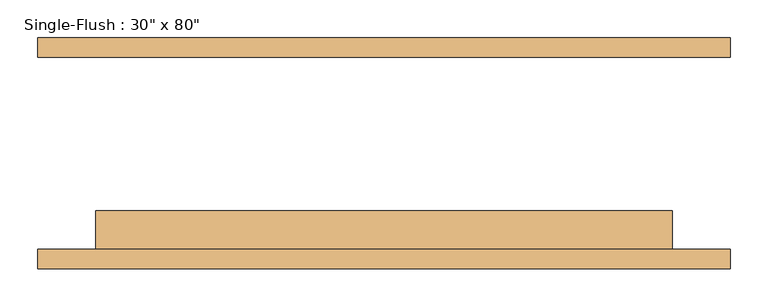
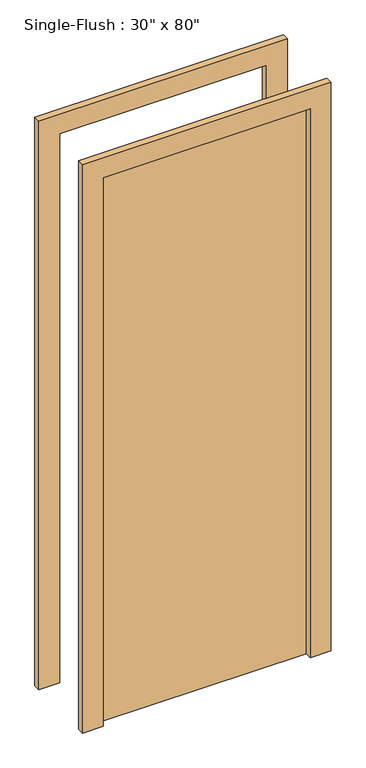
"""IFC4 building model written with IfcOpenShell, lengths in millimetres: door geometry."""

from ifc_helpers import new_model, si_unit, frame, origin, origin_with_axes, place, context, project, spatial, polyline, outline, extrude, source, transform, mapped, element, save


def door_d5d488e1(model_context):
    return source(origin(), model_context, "Body", "SweptSolid", [
        extrude(outline(polyline([(2209.8, -457.2), (0.0, -457.2), (0.0, -381.0), (2133.6, -381.0), (2133.6, 381.0), (0.0, 381.0), (0.0, 457.2), (2209.8, 457.2), (2209.8, -457.2)])), frame((0.0, -152.4, 0.0), z_axis=(0.0, 1.0, 0.0), x_axis=(0.0, 0.0, 1.0)), (0.0, 0.0, 1.0), 25.4),
        extrude(outline(polyline([(2209.8, 457.2), (2209.8, -457.2), (0.0, -457.2), (0.0, -381.0), (2133.6, -381.0), (2133.6, 381.0), (0.0, 381.0), (0.0, 457.2), (2209.8, 457.2)])), frame((0.0, 127.0, 0.0), z_axis=(0.0, 1.0, 0.0), x_axis=(0.0, 0.0, 1.0)), (0.0, 0.0, 1.0), 25.4),
        extrude(outline(polyline([(381.0, -76.2), (381.0, -127.0), (-381.0, -127.0), (-381.0, -76.2), (381.0, -76.2)])), origin_with_axes(), (0.0, 0.0, 1.0), 2133.6),
    ])


if __name__ == "__main__":
    model = new_model("IFC4")
    model_context = context("Model", 3, world=origin())
    ifc_project = project(units=[si_unit("LENGTHUNIT", "METRE", prefix="MILLI")], contexts=[model_context])
    site = spatial("IfcSite", under=ifc_project)
    building = spatial("IfcBuilding", under=site)
    placement = place(None, origin())
    door_shape = door_d5d488e1(model_context)
    element("IfcDoor", 1, ObjectType="Single-Flush : 30\" x 80\"", at=placement, inside=building, context=model_context, shape_type="MappedRepresentation", body=[
        mapped(door_shape, transform((0.0, 0.0, 0.0), x_axis=(1.0, 0.0, 0.0), y_axis=(0.0, 1.0, 0.0), z_axis=(0.0, 0.0, 1.0))),
    ])
    save(model, "model.ifc")

# Revit data of these elements
# Type "Single-Flush : 30\" x 80\""
#   Type Mark = "5"
#   Construction Type Id = "MDOOR"
#   Assembly Code = "C1020"
#   Analytic Construction = "Metal"
#   Thickness = 0' - 2"
#   Heat Transfer Coefficient (U) = 0.651978 BTU/(h·ft²·°F)
#   Height = 7' - 0"
#   Trim Projection Ext = 0' - 1"
#   Trim Projection Int = 0' - 1"
#   Trim Width = 0' - 3"
#   Width = 2' - 6"
#   Define Thermal Properties by = 1
#   Define Thermal Properties by = 1
#   Door Material = Door - Panel
#   Frame Material = Door - Frame
#   Visual Light Transmittance = 0
#   Solar Heat Gain Coefficient = 0
#   Function = (empty or 0)
#   Wall Closure = (empty or 0)
# Element 1 (IfcDoor, "Single-Flush : 30\" x 80\"")
#   Materials on its faces: "Door - Frame", "Door - Panel"
# Materials
#   "Door - Panel": class "Wood", colour RGB 210 159 95, transparency 0, Cost = 0
#   "Door - Frame": colour RGB 118 70 51, transparency 0, Cost = 0
